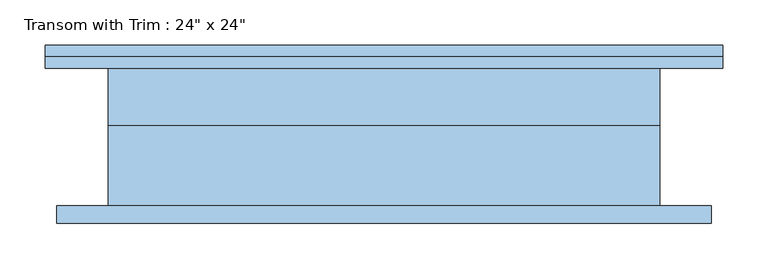
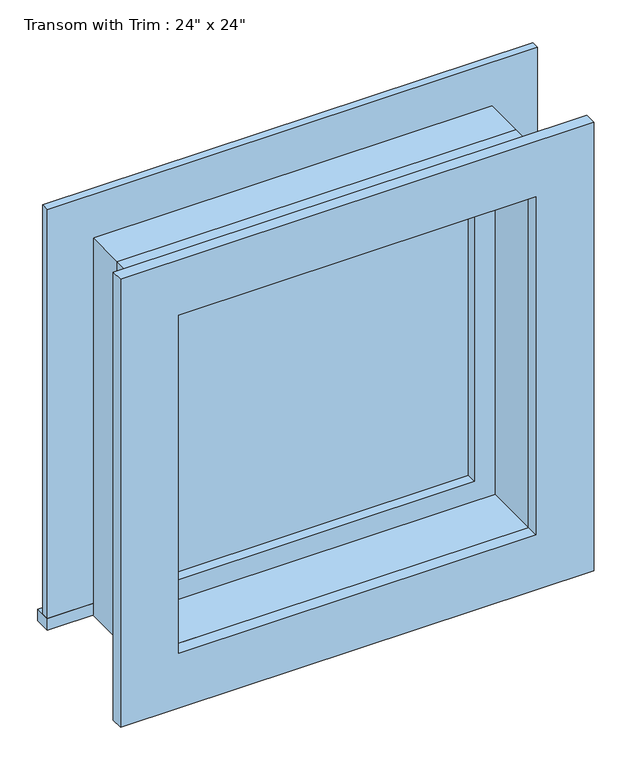
"""IFC4 building model written with IfcOpenShell, lengths in millimetres: window geometry."""

from ifc_helpers import new_model, si_unit, frame, origin, place, context, project, spatial, polyline, outline, extrude, source, transform, mapped, element, save


def window_3d781103(model_context):
    return source(origin(), model_context, "Body", "SweptSolid", [
        extrude(outline(polyline([(-412.75, 101.6), (336.55, 101.6), (336.55, 76.2), (-412.75, 76.2), (-412.75, 101.6)])), frame((0.0, 0.0, 2159.0), z_axis=(0.0, 0.0, 1.0), x_axis=(1.0, 0.0, 0.0)), (0.0, 0.0, 1.0), 19.05),
        extrude(outline(polyline([(2749.55, -323.85), (2749.55, 247.65), (2178.05, 247.65), (2178.05, 336.55), (2838.45, 336.55), (2838.45, -412.75), (2178.05, -412.75), (2178.05, -323.85), (2749.55, -323.85)])), frame((0.0, 76.2, 0.0), z_axis=(0.0, 1.0, 0.0), x_axis=(0.0, 0.0, 1.0)), (0.0, 0.0, 1.0), 12.7),
        extrude(outline(polyline([(2825.75, 323.85), (2825.75, -400.05), (2101.85, -400.05), (2101.85, 323.85), (2825.75, 323.85)]), holes=[polyline([(2736.85, 234.95), (2190.75, 234.95), (2190.75, -311.15), (2736.85, -311.15), (2736.85, 234.95)])]), frame((0.0, -95.25, 0.0), z_axis=(0.0, 1.0, 0.0), x_axis=(0.0, 0.0, 1.0)), (0.0, 0.0, 1.0), 19.05),
        extrude(outline(polyline([(203.2, 28.575), (-279.4, 28.575), (-279.4, 41.275), (203.2, 41.275), (203.2, 28.575)])), frame((0.0, 0.0, 2222.5), z_axis=(0.0, 0.0, 1.0), x_axis=(1.0, 0.0, 0.0)), (0.0, 0.0, 1.0), 482.6),
        extrude(outline(polyline([(2749.55, -323.85), (2178.05, -323.85), (2178.05, 247.65), (2749.55, 247.65), (2749.55, -323.85)]), holes=[polyline([(2705.1, -279.4), (2705.1, 203.2), (2222.5, 203.2), (2222.5, -279.4), (2705.1, -279.4)])]), frame((0.0, 12.7, 0.0), z_axis=(0.0, 1.0, 0.0), x_axis=(0.0, 0.0, 1.0)), (0.0, 0.0, 1.0), 44.45),
        extrude(outline(polyline([(2768.6, -342.9), (2159.0, -342.9), (2159.0, 266.7), (2768.6, 266.7), (2768.6, -342.9)]), holes=[polyline([(2736.85, -311.15), (2736.85, 234.95), (2190.75, 234.95), (2190.75, -311.15), (2736.85, -311.15)])]), frame((0.0, -76.2, 0.0), z_axis=(0.0, 1.0, 0.0), x_axis=(0.0, 0.0, 1.0)), (0.0, 0.0, 1.0), 88.9),
        extrude(outline(polyline([(2768.6, 266.7), (2768.6, -342.9), (2159.0, -342.9), (2159.0, 266.7), (2768.6, 266.7)]), holes=[polyline([(2749.55, 247.65), (2178.05, 247.65), (2178.05, -323.85), (2749.55, -323.85), (2749.55, 247.65)])]), frame((0.0, 12.7, 0.0), z_axis=(0.0, 1.0, 0.0), x_axis=(0.0, 0.0, 1.0)), (0.0, 0.0, 1.0), 63.5),
    ])


if __name__ == "__main__":
    model = new_model("IFC4")
    model_context = context("Model", 3, world=origin())
    ifc_project = project(units=[si_unit("LENGTHUNIT", "METRE", prefix="MILLI")], contexts=[model_context])
    site = spatial("IfcSite", under=ifc_project)
    building = spatial("IfcBuilding", under=site)
    placement = place(None, origin())
    window_shape = window_3d781103(model_context)
    element("IfcWindow", 1, ObjectType="Transom with Trim : 24\" x 24\"", at=placement, inside=building, context=model_context, shape_type="MappedRepresentation", body=[
        mapped(window_shape, transform((0.0, 0.0, 0.0), x_axis=(1.0, 0.0, 0.0), y_axis=(0.0, 1.0, 0.0), z_axis=(0.0, 0.0, 1.0))),
    ])
    save(model, "model.ifc")

# Revit data of these elements
# Type "Transom with Trim : 24\" x 24\""
#   Type Mark = "22"
#   Construction Type Id = "GSP4R"
#   Assembly Code = "B2020100"
#   Analytic Construction = "1/8 in Pilkington single glazing"
#   Visual Light Transmittance = 0.9
#   Solar Heat Gain Coefficient = 0.78
#   Heat Transfer Coefficient (U) = 0.6496 BTU/(h·ft²·°F)
#   Height = 2' - 0"
#   Default Sill Height = 7' - 1"
#   Trim Projection - Ext. = 0' - 0 1/2"
#   Trim Projection - Int. = 0' - 0 3/4"
#   Trim Width - Exterior = 0' - 3 1/2"
#   Trim Width - Interior = 0' - 3 1/2"
#   Width = 2' - 0"
#   Window Inset = 0' - 0 3/4"
#   Define Thermal Properties by = 1
#   Glass Pane Material = Glass
#   Sash Material = Sash
#   Trim Exterior Material = Trim
#   Trim Interior Material = Trim
#   Wall Closure = (empty or 0)
# Element 1 (IfcWindow, "Transom with Trim : 24\" x 24\"")
#   Materials on its faces: "Sash", "Trim", "Glass"
# Materials
#   "Glass": class "Glass", colour RGB 0 128 192, transparency 0.75, Description = "Soda Lime Glass", Cost = 0
#   "Sash": class "Wood", colour RGB 224 178 126, transparency 0
#   "Trim": class "Wood", colour RGB 224 178 126, transparency 0
